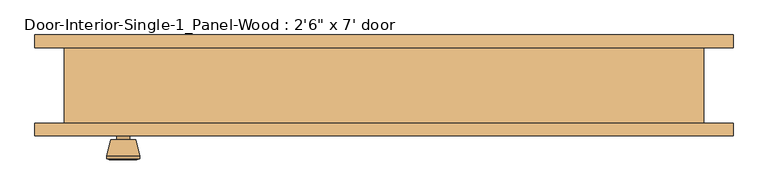
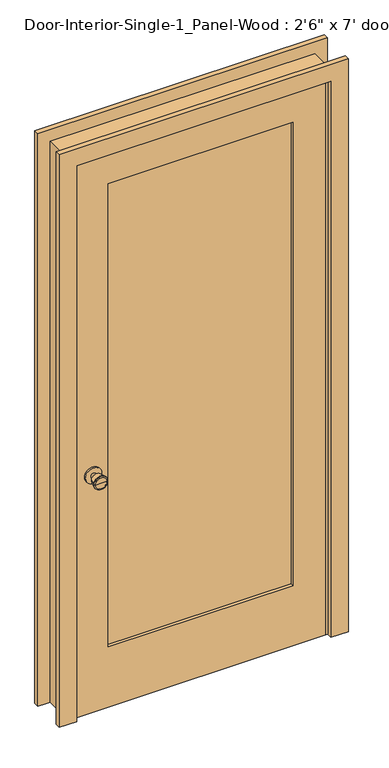
"""IFC4 building model written with IfcOpenShell, lengths in millimetres: door geometry."""

from ifc_helpers import new_model, si_unit, point, frame, frame_2d, origin, place, context, project, spatial, polyline, circle_curve, trimmed, segment, composite_curve, outline, extrude, faceted_brep, source, transform, mapped, element, save
from ifc_brep_helpers import plane_surface, cylinder_surface, revolved_surface, advanced_brep


def door_a3feeac7(model_context):
    return source(origin(), model_context, "Body", "SolidModel", [
        advanced_brep(
        [(-393.7, -13.05, 914.4), (-403.7, -13.05, 914.4), (-383.7, -13.05, 914.4), (-373.2241324, 35.95, 914.4), (-414.1758676, 35.95, 914.4), (-393.7, 35.95, 914.4), (-368.7, 34.1221319, 914.4), (-418.7, 34.1221319, 914.4), (-368.7, 30.6584537, 914.4), (-418.7, 30.6584537, 914.4), (-375.063764, 5.95, 914.4), (-412.336236, 5.95, 914.4), (-383.7, 5.95, 914.4), (-403.7, 5.95, 914.4)],
        [
            (0, 1),
            (1, 2, circle_curve(frame((-393.7, -13.05, 914.4), z_axis=(0.0, -1.0, 0.0), x_axis=(-1.0, 0.0, 0.0)), 10.0)),
            (2, 0),
            (2, 1, circle_curve(frame((-393.7, -13.05, 914.4), z_axis=(0.0, -1.0, 0.0), x_axis=(-1.0, 0.0, 0.0)), 10.0)),
            (3, 4, circle_curve(frame((-393.7, 35.95, 914.4), z_axis=(0.0, 1.0, 0.0), x_axis=(-1.0, 0.0, 0.0)), 20.4758676)),
            (4, 5),
            (5, 3),
            (4, 3, circle_curve(frame((-393.7, 35.95, 914.4), z_axis=(0.0, 1.0, 0.0), x_axis=(-1.0, 0.0, 0.0)), 20.4758676)),
            (6, 7, circle_curve(frame((-393.7, 34.1221319, 914.4), z_axis=(0.0, 1.0, 0.0), x_axis=(-1.0, 0.0, 0.0)), 25.0)),
            (7, 4),
            (3, 6),
            (7, 6, circle_curve(frame((-393.7, 34.1221319, 914.4), z_axis=(0.0, 1.0, 0.0), x_axis=(-1.0, 0.0, 0.0)), 25.0)),
            (8, 9, circle_curve(frame((-393.7, 30.6584537, 914.4), z_axis=(0.0, 1.0, 0.0), x_axis=(-1.0, 0.0, 0.0)), 25.0)),
            (9, 7),
            (6, 8),
            (9, 8, circle_curve(frame((-393.7, 30.6584537, 914.4), z_axis=(0.0, 1.0, 0.0), x_axis=(-1.0, 0.0, 0.0)), 25.0)),
            (10, 11, circle_curve(frame((-393.7, 5.95, 914.4), z_axis=(0.0, 1.0, 0.0), x_axis=(-1.0, 0.0, 0.0)), 18.636236)),
            (11, 9),
            (8, 10),
            (11, 10, circle_curve(frame((-393.7, 5.95, 914.4), z_axis=(0.0, 1.0, 0.0), x_axis=(-1.0, 0.0, 0.0)), 18.636236)),
            (12, 13, circle_curve(frame((-393.7, 5.95, 914.4), z_axis=(0.0, 1.0, 0.0), x_axis=(-1.0, 0.0, 0.0)), 10.0)),
            (13, 11),
            (10, 12),
            (13, 12, circle_curve(frame((-393.7, 5.95, 914.4), z_axis=(0.0, 1.0, 0.0), x_axis=(-1.0, 0.0, 0.0)), 10.0)),
            (1, 13),
            (12, 2),
        ],
        [
            plane_surface(frame((-393.7, -13.05, 914.4), z_axis=(0.0, -1.0, 0.0), x_axis=(-1.0, 0.0, 0.0))),
            plane_surface(frame((-393.7, 35.95, 914.4), z_axis=(0.0, 1.0, 0.0), x_axis=(-1.0, 0.0, 0.0))),
            revolved_surface(polyline([(-414.1758676, 35.95, 914.4), (-418.7, 34.1221319, 914.4)]), (-393.7, -13.05, 914.4), (0.0, -1.0, 0.0)),
            cylinder_surface(frame((-393.7, -13.05, 914.4), z_axis=(0.0, -1.0, 0.0), x_axis=(-1.0, 0.0, 0.0)), 25.0),
            revolved_surface(polyline([(-418.7, 30.6584537, 914.4), (-412.336236, 5.95, 914.4)]), (-393.7, -13.05, 914.4), (0.0, -1.0, 0.0)),
            plane_surface(frame((-393.7, 5.95, 914.4), z_axis=(0.0, -1.0, 0.0), x_axis=(-1.0, 0.0, 0.0))),
            cylinder_surface(frame((-393.7, -13.05, 914.4), z_axis=(0.0, -1.0, 0.0), x_axis=(-1.0, 0.0, 0.0)), 10.0),
        ],
        [
            (0, [[1, 2, 3]]),
            (0, [[-3, 4, -1]]),
            (1, [[5, 6, 7]]),
            (1, [[8, -7, -6]]),
            (2, [[9, 10, -5, 11]]),
            (2, [[12, -11, -8, -10]]),
            (3, [[13, 14, -9, 15]]),
            (3, [[16, -15, -12, -14]]),
            (4, [[17, 18, -13, 19]]),
            (4, [[20, -19, -16, -18]]),
            (5, [[21, 22, -17, 23]]),
            (5, [[24, -23, -20, -22]]),
            (6, [[-2, 25, -21, 26]]),
            (6, [[-4, -26, -24, -25]]),
        ],
    ),
        extrude(outline(composite_curve([segment(trimmed(circle_curve(frame_2d((914.4, -393.7)), 30.0), [point((914.4, -423.7))], [point((914.4, -363.7))], False, "CARTESIAN"), True, "CONTINUOUS"), segment(trimmed(circle_curve(frame_2d((914.4, -393.7)), 30.0), [point((914.4, -363.7))], [point((914.4, -423.7))], False, "CARTESIAN"), True, "CONTINUOUS")], self_intersect=False)), frame((0.0, -19.05, 0.0), z_axis=(0.0, 1.0, 0.0), x_axis=(0.0, 0.0, 1.0)), (0.0, 0.0, 1.0), 6.0),
        advanced_brep(
        [(-393.7, -59.975, 914.4), (-383.7, -59.975, 914.4), (-403.7, -59.975, 914.4), (-373.2241324, -108.975, 914.4), (-393.7, -108.975, 914.4), (-414.1758676, -108.975, 914.4), (-368.7, -107.1471319, 914.4), (-418.7, -107.1471319, 914.4), (-368.7, -103.6834537, 914.4), (-418.7, -103.6834537, 914.4), (-375.063764, -78.975, 914.4), (-412.336236, -78.975, 914.4), (-383.7, -78.975, 914.4), (-403.7, -78.975, 914.4)],
        [
            (0, 1),
            (1, 2, circle_curve(frame((-393.7, -59.975, 914.4), z_axis=(0.0, 1.0, 0.0), x_axis=(-1.0, 0.0, 0.0)), 10.0)),
            (2, 0),
            (2, 1, circle_curve(frame((-393.7, -59.975, 914.4), z_axis=(0.0, 1.0, 0.0), x_axis=(-1.0, 0.0, 0.0)), 10.0)),
            (3, 4),
            (4, 5),
            (5, 3, circle_curve(frame((-393.7, -108.975, 914.4), z_axis=(0.0, -1.0, 0.0), x_axis=(-1.0, 0.0, 0.0)), 20.4758676)),
            (3, 5, circle_curve(frame((-393.7, -108.975, 914.4), z_axis=(0.0, -1.0, 0.0), x_axis=(-1.0, 0.0, 0.0)), 20.4758676)),
            (6, 3),
            (5, 7),
            (7, 6, circle_curve(frame((-393.7, -107.1471319, 914.4), z_axis=(0.0, -1.0, 0.0), x_axis=(-1.0, 0.0, 0.0)), 25.0)),
            (6, 7, circle_curve(frame((-393.7, -107.1471319, 914.4), z_axis=(0.0, -1.0, 0.0), x_axis=(-1.0, 0.0, 0.0)), 25.0)),
            (8, 6),
            (7, 9),
            (9, 8, circle_curve(frame((-393.7, -103.6834537, 914.4), z_axis=(0.0, -1.0, 0.0), x_axis=(-1.0, 0.0, 0.0)), 25.0)),
            (8, 9, circle_curve(frame((-393.7, -103.6834537, 914.4), z_axis=(0.0, -1.0, 0.0), x_axis=(-1.0, 0.0, 0.0)), 25.0)),
            (10, 8),
            (9, 11),
            (11, 10, circle_curve(frame((-393.7, -78.975, 914.4), z_axis=(0.0, -1.0, 0.0), x_axis=(-1.0, 0.0, 0.0)), 18.636236)),
            (10, 11, circle_curve(frame((-393.7, -78.975, 914.4), z_axis=(0.0, -1.0, 0.0), x_axis=(-1.0, 0.0, 0.0)), 18.636236)),
            (12, 10),
            (11, 13),
            (13, 12, circle_curve(frame((-393.7, -78.975, 914.4), z_axis=(0.0, -1.0, 0.0), x_axis=(-1.0, 0.0, 0.0)), 10.0)),
            (12, 13, circle_curve(frame((-393.7, -78.975, 914.4), z_axis=(0.0, -1.0, 0.0), x_axis=(-1.0, 0.0, 0.0)), 10.0)),
            (1, 12),
            (13, 2),
        ],
        [
            plane_surface(frame((-393.7, -59.975, 914.4), z_axis=(0.0, 1.0, 0.0), x_axis=(-1.0, 0.0, 0.0))),
            plane_surface(frame((-393.7, -108.975, 914.4), z_axis=(0.0, -1.0, 0.0), x_axis=(-1.0, 0.0, 0.0))),
            revolved_surface(polyline([(-414.1758676, -108.975, 914.4), (-418.7, -107.1471319, 914.4)]), (-393.7, -59.975, 914.4), (0.0, 1.0, 0.0)),
            cylinder_surface(frame((-393.7, -59.975, 914.4), z_axis=(0.0, 1.0, 0.0), x_axis=(-1.0, 0.0, 0.0)), 25.0),
            revolved_surface(polyline([(-418.7, -103.6834537, 914.4), (-412.336236, -78.975, 914.4)]), (-393.7, -59.975, 914.4), (0.0, 1.0, 0.0)),
            plane_surface(frame((-393.7, -78.975, 914.4), z_axis=(0.0, 1.0, 0.0), x_axis=(-1.0, 0.0, 0.0))),
            cylinder_surface(frame((-393.7, -59.975, 914.4), z_axis=(0.0, 1.0, 0.0), x_axis=(-1.0, 0.0, 0.0)), 10.0),
        ],
        [
            (0, [[1, 2, 3]]),
            (0, [[-3, 4, -1]]),
            (1, [[5, 6, 7]]),
            (1, [[-6, -5, 8]]),
            (2, [[9, -7, 10, 11]]),
            (2, [[-10, -8, -9, 12]]),
            (3, [[13, -11, 14, 15]]),
            (3, [[-14, -12, -13, 16]]),
            (4, [[17, -15, 18, 19]]),
            (4, [[-18, -16, -17, 20]]),
            (5, [[21, -19, 22, 23]]),
            (5, [[-22, -20, -21, 24]]),
            (6, [[25, -23, 26, -2]]),
            (6, [[-26, -24, -25, -4]]),
        ],
    ),
        extrude(outline(composite_curve([segment(trimmed(circle_curve(frame_2d((914.4, -393.7)), 30.0), [point((914.4, -423.7))], [point((914.4, -363.7))], False, "CARTESIAN"), True, "CONTINUOUS"), segment(trimmed(circle_curve(frame_2d((914.4, -393.7)), 30.0), [point((914.4, -363.7))], [point((914.4, -423.7))], False, "CARTESIAN"), True, "CONTINUOUS")], self_intersect=False)), frame((0.0, -59.975, 0.0), z_axis=(0.0, 1.0, 0.0), x_axis=(0.0, 0.0, 1.0)), (0.0, 0.0, 1.0), 6.0),
        faceted_brep([(482.6, -53.975, 0.0), (457.2, -53.975, 0.0), (457.2, -19.05, 0.0), (444.5, -19.05, 0.0), (444.5, 15.875, 0.0), (457.2, 15.875, 0.0), (457.2, 60.325, 0.0), (482.6, 60.325, 0.0), (482.6, 60.325, 2159.0), (482.6, -53.975, 2159.0), (457.2, 60.325, 2133.6), (-457.2, 60.325, 2133.6), (-457.2, 60.325, 0.0), (-482.6, 60.325, 0.0), (-482.6, 60.325, 2159.0), (457.2, 15.875, 2133.6), (444.5, 15.875, 2120.9), (-444.5, 15.875, 2120.9), (-444.5, 15.875, 0.0), (-457.2, 15.875, 0.0), (-457.2, 15.875, 2133.6), (444.5, -19.05, 2120.9), (457.2, -19.05, 2133.6), (-457.2, -19.05, 2133.6), (-457.2, -19.05, 0.0), (-444.5, -19.05, 0.0), (-444.5, -19.05, 2120.9), (457.2, -53.975, 2133.6), (-482.6, -53.975, 2159.0), (-482.6, -53.975, 0.0), (-457.2, -53.975, 0.0), (-457.2, -53.975, 2133.6)], [[[0, 1, 2, 3, 4, 5, 6, 7]], [[7, 8, 9, 0]], [[6, 10, 11, 12, 13, 14, 8, 7]], [[5, 15, 10, 6]], [[4, 16, 17, 18, 19, 20, 15, 5]], [[3, 21, 16, 4]], [[2, 22, 23, 24, 25, 26, 21, 3]], [[1, 27, 22, 2]], [[0, 9, 28, 29, 30, 31, 27, 1]], [[8, 14, 28, 9]], [[15, 20, 11, 10]], [[21, 26, 17, 16]], [[27, 31, 23, 22]], [[29, 13, 12, 19, 18, 25, 24, 30]], [[14, 13, 29, 28]], [[20, 19, 12, 11]], [[26, 25, 18, 17]], [[31, 30, 24, 23]]]),
        extrude(outline(polyline([(2133.6, -457.2), (0.0, -457.2), (0.0, 457.2), (2133.6, 457.2), (2133.6, -457.2)]), holes=[polyline([(2014.5375, -336.55), (2014.5375, 336.55), (231.775, 336.55), (231.775, -336.55), (2014.5375, -336.55)])]), frame((0.0, -53.975, 0.0), z_axis=(0.0, 1.0, 0.0), x_axis=(0.0, 0.0, 1.0)), (0.0, 0.0, 1.0), 34.925),
        extrude(outline(polyline([(336.55, -30.6916667), (336.55, -42.3333333), (-336.55, -42.3333333), (-336.55, -30.6916667), (336.55, -30.6916667)])), frame((0.0, 0.0, 231.775), z_axis=(0.0, 0.0, 1.0), x_axis=(1.0, 0.0, 0.0)), (0.0, 0.0, 1.0), 1782.7625),
        extrude(outline(polyline([(0.0, 527.05), (2203.45, 527.05), (2203.45, -527.05), (0.0, -527.05), (0.0, -463.55), (2139.95, -463.55), (2139.95, 463.55), (0.0, 463.55), (0.0, 527.05)])), frame((0.0, -73.025, 0.0), z_axis=(0.0, 1.0, 0.0), x_axis=(0.0, 0.0, 1.0)), (0.0, 0.0, 1.0), 19.05),
        extrude(outline(polyline([(0.0, 527.05), (2203.45, 527.05), (2203.45, -527.05), (0.0, -527.05), (0.0, -463.55), (2139.95, -463.55), (2139.95, 463.55), (0.0, 463.55), (0.0, 527.05)])), frame((0.0, 60.325, 0.0), z_axis=(0.0, 1.0, 0.0), x_axis=(0.0, 0.0, 1.0)), (0.0, 0.0, 1.0), 19.05),
    ])


if __name__ == "__main__":
    model = new_model("IFC4")
    model_context = context("Model", 3, world=origin())
    ifc_project = project(units=[si_unit("LENGTHUNIT", "METRE", prefix="MILLI")], contexts=[model_context])
    site = spatial("IfcSite", under=ifc_project)
    building = spatial("IfcBuilding", under=site)
    placement = place(None, origin())
    door_shape = door_a3feeac7(model_context)
    element("IfcDoor", 1, ObjectType="Door-Interior-Single-1_Panel-Wood : 2'6\" x 7' door", at=placement, inside=building, context=model_context, shape_type="MappedRepresentation", body=[
        mapped(door_shape, transform((0.0, 0.0, 0.0), x_axis=(1.0, 0.0, 0.0), y_axis=(0.0, 1.0, 0.0), z_axis=(0.0, 0.0, 1.0))),
    ])
    save(model, "model.ifc")

# Revit data of these elements
# Type "Door-Interior-Single-1_Panel-Wood : 2'6\" x 7' door"
#   Type Mark = "9"
#   Assembly Code = "C1020300"
#   Analytic Construction = "Wooden"
#   Top Rail = 0' - 4 11/16"
#   Thickness = 0' - 1 3/8"
#   Thermal Resistance (R) = 2.5876 (h·ft²·°F)/BTU
#   Swing Angle [instance default] = 90.00°
#   Stiles = 0' - 4 3/4"
#   Rough Width = 3' - 2"
#   Rough Height = 7' - 1"
#   Height = 7' - 0"
#   Width = 3' - 0"
#   Heat Transfer Coefficient (U) = 0.3865 BTU/(h·ft²·°F)
#   Bottom Rail = 0' - 9 1/8"
#   Trim Material = Cherry
#   Panel Material = Cherry
#   Frame Material = Cherry
#   Door Handle Material = Aluminum
#   Visual Light Transmittance = 0
#   Solar Heat Gain Coefficient = 0
#   Wall Closure = (empty or 0)
#   Function = (empty or 0)
# Element 1 (IfcDoor, "Door-Interior-Single-1_Panel-Wood : 2'6\" x 7' door")
#   Materials on its faces: "Cherry", "Aluminum"
# Materials
#   "Cherry": class "Wood", colour RGB 226 177 128, transparency 0, Description = "Prunus Serotina", Cost = 0
#   "Aluminum": class "Metal", colour RGB 247 247 247, transparency 0, Description = "Aluminum 6061", Cost = 0
